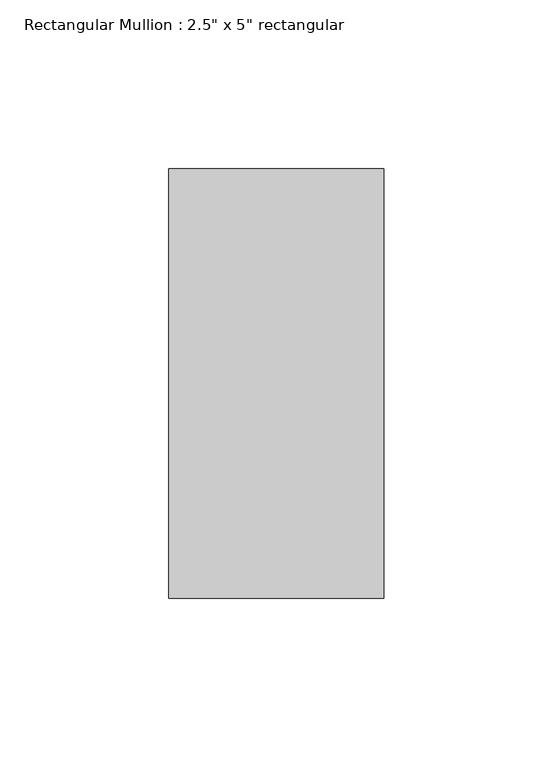
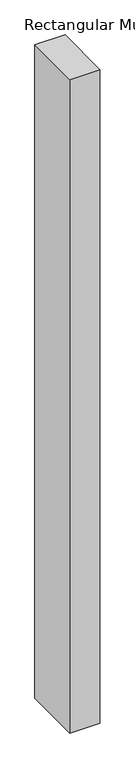
"""IFC4 building model written with IfcOpenShell, lengths in millimetres: member geometry."""

from ifc_helpers import new_model, si_unit, frame, origin, place, context, project, spatial, polyline, outline, extrude, source, transform, mapped, element, save


def member_141a309f(model_context):
    return source(origin(), model_context, "Body", "SweptSolid", [
        extrude(outline(polyline([(31.75, 63.5), (31.75, -63.5), (-31.75, -63.5), (-31.75, 63.5), (31.75, 63.5)])), frame((0.0, 0.0, -1452.5193485), z_axis=(0.0, 0.0, 1.0), x_axis=(1.0, 0.0, 0.0)), (0.0, 0.0, 1.0), 1452.5193485),
    ])


if __name__ == "__main__":
    model = new_model("IFC4")
    model_context = context("Model", 3, world=origin())
    ifc_project = project(units=[si_unit("LENGTHUNIT", "METRE", prefix="MILLI")], contexts=[model_context])
    site = spatial("IfcSite", under=ifc_project)
    building = spatial("IfcBuilding", under=site)
    placement = place(None, origin())
    member_shape = member_141a309f(model_context)
    element("IfcMember", 1, ObjectType="Rectangular Mullion : 2.5\" x 5\" rectangular", at=placement, inside=building, context=model_context, shape_type="MappedRepresentation", body=[
        mapped(member_shape, transform((0.0, 0.0, 0.0), x_axis=(1.0, 0.0, 0.0), y_axis=(0.0, 1.0, 0.0), z_axis=(0.0, 0.0, 1.0))),
    ])
    save(model, "model.ifc")

# Revit data of these elements
# Type "Rectangular Mullion : 2.5\" x 5\" rectangular"
#   built-in parameter 1007304 = 0.416667 (stored number, unit not read)
#   built-in parameter 1007301 = 0.104167 (stored number, unit not read)
#   built-in parameter 1007300 = 0.104167 (stored number, unit not read)
# Element 1 (IfcMember, "Rectangular Mullion : 2.5\" x 5\" rectangular")
#   Materials on its faces: "Aluminum"
# Materials
#   "Aluminum": class "Metal", colour RGB 247 247 247, transparency 0, Description = "Aluminum 6061", Cost = 0
